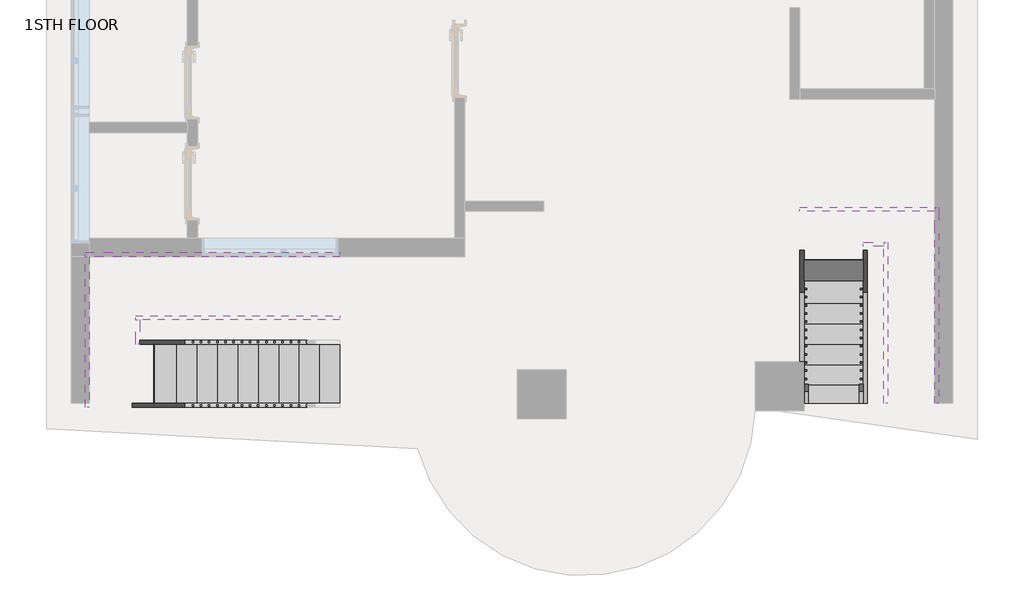
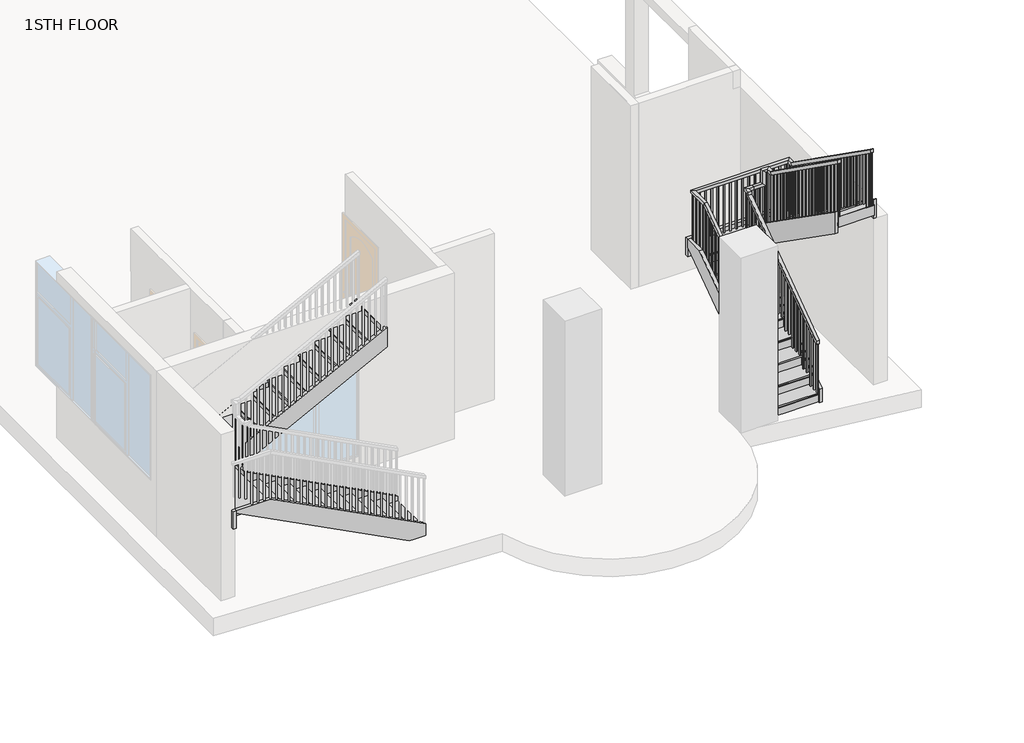
# One storey, part 4 of 4: 12 members, 2 railings, 2 stair flights.
"""IFC4 building model written with IfcOpenShell, lengths in millimetres."""

from ifc_helpers import new_model, si_unit, frame, origin, place, context, project, spatial, polyline, outline, extrude, faceted_brep, transform, mapped, element, save
from components import stair_flight_8de044e6, stair_flight_1dbbfd26

model = new_model("IFC4")

# Units and contexts
model_context = context("Model", 3, world=origin())
ifc_project = project(units=[si_unit("LENGTHUNIT", "METRE", prefix="MILLI")], contexts=[model_context])

# Site, building, storey
site = spatial("IfcSite", under=ifc_project)
building = spatial("IfcBuilding", under=site)
storey = spatial("IfcBuildingStorey", under=building, Name="1STH FLOOR", Elevation=3200.4)

# Members
placement = place(None, origin())
element("IfcMember", 1, ObjectType="Stringer - 2\" Width", at=placement, inside=storey, context=model_context, shape_type="SweptSolid", body=[
    extrude(outline(polyline([(3200.4, -3117.2664982), (3404.9197081, -3117.2664982), (4724.4, -5663.6319738), (4724.4, -6232.5131972), (4675.8929835, -6232.5131972), (3200.4, -3385.0705974), (3200.4, -3117.2664982)])), frame((0.0, -7701.7822004, 0.0), z_axis=(0.0, 1.0, 0.0), x_axis=(0.0, 0.0, 1.0)), (0.0, 0.0, 1.0), 50.8),
])
element("IfcMember", 2, ObjectType="Stringer - 2\" Width", at=placement, inside=storey, context=model_context, shape_type="SweptSolid", body=[
    extrude(outline(polyline([(-6232.5131972, -7701.7822004), (-6283.3131972, -7701.7822004), (-6283.3131972, -5824.7082131), (-6232.5131972, -5824.7082131), (-6232.5131972, -7701.7822004)])), frame((0.0, 0.0, 4419.6), z_axis=(0.0, 0.0, 1.0), x_axis=(1.0, 0.0, 0.0)), (0.0, 0.0, 1.0), 304.8),
])
element("IfcMember", 3, ObjectType="Stringer - 2\" Width", at=placement, inside=storey, context=model_context, shape_type="SweptSolid", body=[
    extrude(outline(polyline([(4528.3136913, -6283.3131972), (4419.6, -6283.3131972), (4419.6, -5830.6202937), (5825.6106031, -3117.2664982), (6168.9015263, -3117.2664982), (4528.3136913, -6283.3131972)])), frame((0.0, -5824.7082131, 0.0), z_axis=(0.0, 1.0, 0.0), x_axis=(0.0, 0.0, 1.0)), (0.0, 0.0, 1.0), 50.8),
])
element("IfcMember", 4, ObjectType="Stringer - 2\" Width", at=placement, inside=storey, context=model_context, shape_type="SweptSolid", body=[
    extrude(outline(polyline([(3200.4, -3117.2664982), (3404.9197081, -3117.2664982), (4694.7778899, -5606.4664982), (4351.4869668, -5606.4664982), (3200.4, -3385.0705974), (3200.4, -3117.2664982)])), frame((0.0, -6914.3822004, 0.0), z_axis=(0.0, 1.0, 0.0), x_axis=(0.0, 0.0, 1.0)), (0.0, 0.0, 1.0), 50.8),
])
element("IfcMember", 5, ObjectType="Stringer - 2\" Width", at=placement, inside=storey, context=model_context, shape_type="SweptSolid", body=[
    extrude(outline(polyline([(-5606.4664982, -6914.3822004), (-5657.2664982, -6914.3822004), (-5657.2664982, -6609.5822004), (-5606.4664982, -6609.5822004), (-5606.4664982, -6914.3822004)])), frame((0.0, 0.0, 4419.6), z_axis=(0.0, 0.0, 1.0), x_axis=(1.0, 0.0, 0.0)), (0.0, 0.0, 1.0), 304.8),
])
element("IfcMember", 6, ObjectType="Stringer - 2\" Width", at=placement, inside=storey, context=model_context, shape_type="SweptSolid", body=[
    extrude(outline(polyline([(4852.7197081, -5657.2664982), (4509.4287849, -5657.2664982), (5825.6106031, -3117.2664982), (6168.9015263, -3117.2664982), (4852.7197081, -5657.2664982)])), frame((0.0, -6609.5822004, 0.0), z_axis=(0.0, 1.0, 0.0), x_axis=(0.0, 0.0, 1.0)), (0.0, 0.0, 1.0), 50.8),
])
element("IfcMember", 7, ObjectType="Stringer - 2\" Width", at=placement, inside=storey, context=model_context, shape_type="SweptSolid", body=[
    extrude(outline(polyline([(-7650.9822004, 3200.4), (-7650.9822004, 3439.699187), (-5597.981039, 4876.8), (-5263.3822004, 4876.8), (-5263.3822004, 4738.9633718), (-7461.3298744, 3200.4), (-7650.9822004, 3200.4)])), frame((2606.6891134, 0.0, 0.0), z_axis=(1.0, 0.0, 0.0), x_axis=(0.0, 1.0, 0.0)), (0.0, 0.0, 1.0), 50.8),
])
element("IfcMember", 8, ObjectType="Stringer - 2\" Width", at=placement, inside=storey, context=model_context, shape_type="SweptSolid", body=[
    extrude(outline(polyline([(2606.6891134, -5263.3822004), (2606.6891134, -5212.5822004), (4281.7311655, -5212.5822004), (4281.7311655, -5263.3822004), (2606.6891134, -5263.3822004)])), frame((0.0, 0.0, 4572.0), z_axis=(0.0, 0.0, 1.0), x_axis=(1.0, 0.0, 0.0)), (0.0, 0.0, 1.0), 304.8),
])
element("IfcMember", 9, ObjectType="Stringer - 2\" Width", at=placement, inside=storey, context=model_context, shape_type="SweptSolid", body=[
    extrude(outline(polyline([(-5212.5822004, 4719.859187), (-5212.5822004, 4572.0), (-5532.8630978, 4572.0), (-7650.9822004, 6054.6833718), (-7650.9822004, 6426.739187), (-5212.5822004, 4719.859187)])), frame((4281.7311655, 0.0, 0.0), z_axis=(1.0, 0.0, 0.0), x_axis=(0.0, 1.0, 0.0)), (0.0, 0.0, 1.0), 50.8),
])
element("IfcMember", 10, ObjectType="Stringer - 2\" Width", at=placement, inside=storey, context=model_context, shape_type="SweptSolid", body=[
    extrude(outline(polyline([(-7650.9822004, 3200.4), (-7650.9822004, 3439.699187), (-5695.1822004, 4808.759187), (-5695.1822004, 4436.7033718), (-7461.3298744, 3200.4), (-7650.9822004, 3200.4)])), frame((3394.0891134, 0.0, 0.0), z_axis=(1.0, 0.0, 0.0), x_axis=(0.0, 1.0, 0.0)), (0.0, 0.0, 1.0), 50.8),
])
element("IfcMember", 11, ObjectType="Stringer - 2\" Width", at=placement, inside=storey, context=model_context, shape_type="SweptSolid", body=[
    extrude(outline(polyline([(3394.0891134, -5695.1822004), (3394.0891134, -5644.3822004), (3648.0891134, -5644.3822004), (3648.0891134, -5695.1822004), (3394.0891134, -5695.1822004)])), frame((0.0, 0.0, 4572.0), z_axis=(0.0, 0.0, 1.0), x_axis=(1.0, 0.0, 0.0)), (0.0, 0.0, 1.0), 304.8),
])
element("IfcMember", 12, ObjectType="Stringer - 2\" Width", at=placement, inside=storey, context=model_context, shape_type="SweptSolid", body=[
    extrude(outline(polyline([(-5644.3822004, 5022.119187), (-5644.3822004, 4650.0633718), (-7650.9822004, 6054.6833718), (-7650.9822004, 6426.739187), (-5644.3822004, 5022.119187)])), frame((3648.0891134, 0.0, 0.0), z_axis=(1.0, 0.0, 0.0), x_axis=(0.0, 1.0, 0.0)), (0.0, 0.0, 1.0), 50.8),
])

# Railings
element("IfcRailing", 13, ObjectType="Handrail - Rectangular", at=placement, inside=storey, context=model_context, shape_type="SolidModel", body=[
    faceted_brep([(3343.2891134, -7650.9822004, 4292.6), (3343.2891134, -7650.9822004, 4230.3314749), (3394.0891134, -7650.9822004, 4230.3314749), (3394.0891134, -7650.9822004, 4292.6), (3343.2891134, -5720.5822004, 5660.9848101), (3343.2891134, -5669.7822004, 5634.7264116), (3394.0891134, -5669.7822004, 5634.7264116), (3394.0891134, -5720.5822004, 5660.9848101), (3343.2891134, -5720.5822004, 5715.0), (3343.2891134, -5669.7822004, 5664.2), (3394.0891134, -5669.7822004, 5664.2), (3394.0891134, -5720.5822004, 5715.0), (3343.2891134, -5593.5822004, 5715.0), (3343.2891134, -5593.5822004, 5664.2), (3394.0891134, -5644.3822004, 5664.2), (3394.0891134, -5644.3822004, 5715.0), (3470.2891134, -5593.5822004, 5715.0), (3470.2891134, -5593.5822004, 5664.2), (3470.2891134, -5644.3822004, 5664.2), (3470.2891134, -5644.3822004, 5715.0), (3622.6891134, -5593.5822004, 5715.0), (3673.4891134, -5593.5822004, 5664.2), (3673.4891134, -5644.3822004, 5664.2), (3622.6891134, -5644.3822004, 5715.0), (3622.6891134, -5593.5822004, 5946.8151899), (3673.4891134, -5593.5822004, 5896.0151899), (3673.4891134, -5644.3822004, 5896.0151899), (3622.6891134, -5644.3822004, 5946.8151899), (3749.6891134, -5593.5822004, 5946.8151899), (3749.6891134, -5593.5822004, 5896.0151899), (3698.8891134, -5644.3822004, 5896.0151899), (3698.8891134, -5644.3822004, 5946.8151899), (3749.6891134, -5720.5822004, 5946.8151899), (3749.6891134, -5736.7610126, 5896.0151899), (3698.8891134, -5736.7610126, 5896.0151899), (3698.8891134, -5720.5822004, 5946.8151899), (3749.6891134, -7650.9822004, 7315.2), (3698.8891134, -7650.9822004, 7315.2), (3698.8891134, -7650.9822004, 7252.9314749), (3749.6891134, -7650.9822004, 7252.9314749)], [[[0, 1, 2, 3]], [[1, 0, 4, 5]], [[2, 1, 5, 6]], [[3, 2, 6, 7]], [[0, 3, 7, 4]], [[5, 4, 8, 9]], [[6, 5, 9, 10]], [[7, 6, 10, 11]], [[4, 7, 11, 8]], [[9, 8, 12, 13]], [[10, 9, 13, 14]], [[11, 10, 14, 15]], [[8, 11, 15, 12]], [[13, 12, 16, 17]], [[14, 13, 17, 18]], [[15, 14, 18, 19]], [[12, 15, 19, 16]], [[17, 16, 20, 21]], [[18, 17, 21, 22]], [[19, 18, 22, 23]], [[16, 19, 23, 20]], [[21, 20, 24, 25]], [[22, 21, 25, 26]], [[23, 22, 26, 27]], [[20, 23, 27, 24]], [[25, 24, 28, 29]], [[26, 25, 29, 30]], [[27, 26, 30, 31]], [[24, 27, 31, 28]], [[29, 28, 32, 33]], [[30, 29, 33, 34]], [[31, 30, 34, 35]], [[28, 31, 35, 32]], [[36, 37, 38, 39]], [[33, 32, 36, 39]], [[34, 33, 39, 38]], [[35, 34, 38, 37]], [[32, 35, 37, 36]]]),
    extrude(outline(polyline([(-7558.9072004, 7187.6631205), (-7539.8572004, 7174.159323), (-7539.8572004, 6223.0), (-7558.9072004, 6223.0), (-7558.9072004, 7187.6631205)])), frame((3714.7641134, 0.0, 0.0), z_axis=(1.0, 0.0, 0.0), x_axis=(0.0, 1.0, 0.0)), (0.0, 0.0, 1.0), 19.05),
    extrude(outline(polyline([(-7457.3072004, 7115.6428673), (-7438.2572004, 7102.1390699), (-7438.2572004, 6223.0), (-7457.3072004, 6223.0), (-7457.3072004, 7115.6428673)])), frame((3714.7641134, 0.0, 0.0), z_axis=(1.0, 0.0, 0.0), x_axis=(0.0, 1.0, 0.0)), (0.0, 0.0, 1.0), 19.05),
    extrude(outline(polyline([(-7355.7072004, 7043.6226142), (-7336.6572004, 7030.1188167), (-7336.6572004, 6045.2), (-7355.7072004, 6045.2), (-7355.7072004, 7043.6226142)])), frame((3714.7641134, 0.0, 0.0), z_axis=(1.0, 0.0, 0.0), x_axis=(0.0, 1.0, 0.0)), (0.0, 0.0, 1.0), 19.05),
    extrude(outline(polyline([(-7254.1072004, 6971.602361), (-7235.0572004, 6958.0985635), (-7235.0572004, 6045.2), (-7254.1072004, 6045.2), (-7254.1072004, 6971.602361)])), frame((3714.7641134, 0.0, 0.0), z_axis=(1.0, 0.0, 0.0), x_axis=(0.0, 1.0, 0.0)), (0.0, 0.0, 1.0), 19.05),
    extrude(outline(polyline([(-7152.5072004, 6899.5821078), (-7133.4572004, 6886.0783104), (-7133.4572004, 5867.4), (-7152.5072004, 5867.4), (-7152.5072004, 6899.5821078)])), frame((3714.7641134, 0.0, 0.0), z_axis=(1.0, 0.0, 0.0), x_axis=(0.0, 1.0, 0.0)), (0.0, 0.0, 1.0), 19.05),
    extrude(outline(polyline([(-7050.9072004, 6827.5618547), (-7031.8572004, 6814.0580572), (-7031.8572004, 5867.4), (-7050.9072004, 5867.4), (-7050.9072004, 6827.5618547)])), frame((3714.7641134, 0.0, 0.0), z_axis=(1.0, 0.0, 0.0), x_axis=(0.0, 1.0, 0.0)), (0.0, 0.0, 1.0), 19.05),
    extrude(outline(polyline([(-6949.3072004, 6755.5416015), (-6930.2572004, 6742.037804), (-6930.2572004, 5867.4), (-6949.3072004, 5867.4), (-6949.3072004, 6755.5416015)])), frame((3714.7641134, 0.0, 0.0), z_axis=(1.0, 0.0, 0.0), x_axis=(0.0, 1.0, 0.0)), (0.0, 0.0, 1.0), 19.05),
    extrude(outline(polyline([(-6847.7072004, 6683.5213483), (-6828.6572004, 6670.0175509), (-6828.6572004, 5689.6), (-6847.7072004, 5689.6), (-6847.7072004, 6683.5213483)])), frame((3714.7641134, 0.0, 0.0), z_axis=(1.0, 0.0, 0.0), x_axis=(0.0, 1.0, 0.0)), (0.0, 0.0, 1.0), 19.05),
    extrude(outline(polyline([(-6746.1072004, 6611.5010952), (-6727.0572004, 6597.9972977), (-6727.0572004, 5689.6), (-6746.1072004, 5689.6), (-6746.1072004, 6611.5010952)])), frame((3714.7641134, 0.0, 0.0), z_axis=(1.0, 0.0, 0.0), x_axis=(0.0, 1.0, 0.0)), (0.0, 0.0, 1.0), 19.05),
    extrude(outline(polyline([(-6644.5072004, 6539.480842), (-6625.4572004, 6525.9770445), (-6625.4572004, 5511.8), (-6644.5072004, 5511.8), (-6644.5072004, 6539.480842)])), frame((3714.7641134, 0.0, 0.0), z_axis=(1.0, 0.0, 0.0), x_axis=(0.0, 1.0, 0.0)), (0.0, 0.0, 1.0), 19.05),
    extrude(outline(polyline([(-6542.9072004, 6467.4605888), (-6523.8572004, 6453.9567914), (-6523.8572004, 5511.8), (-6542.9072004, 5511.8), (-6542.9072004, 6467.4605888)])), frame((3714.7641134, 0.0, 0.0), z_axis=(1.0, 0.0, 0.0), x_axis=(0.0, 1.0, 0.0)), (0.0, 0.0, 1.0), 19.05),
    extrude(outline(polyline([(-6441.3072004, 6395.4403357), (-6422.2572004, 6381.9365382), (-6422.2572004, 5511.8), (-6441.3072004, 5511.8), (-6441.3072004, 6395.4403357)])), frame((3714.7641134, 0.0, 0.0), z_axis=(1.0, 0.0, 0.0), x_axis=(0.0, 1.0, 0.0)), (0.0, 0.0, 1.0), 19.05),
    extrude(outline(polyline([(-6339.7072004, 6323.4200825), (-6320.6572004, 6309.916285), (-6320.6572004, 5334.0), (-6339.7072004, 5334.0), (-6339.7072004, 6323.4200825)])), frame((3714.7641134, 0.0, 0.0), z_axis=(1.0, 0.0, 0.0), x_axis=(0.0, 1.0, 0.0)), (0.0, 0.0, 1.0), 19.05),
    extrude(outline(polyline([(-6238.1072004, 6251.3998293), (-6219.0572004, 6237.8960319), (-6219.0572004, 5334.0), (-6238.1072004, 5334.0), (-6238.1072004, 6251.3998293)])), frame((3714.7641134, 0.0, 0.0), z_axis=(1.0, 0.0, 0.0), x_axis=(0.0, 1.0, 0.0)), (0.0, 0.0, 1.0), 19.05),
    extrude(outline(polyline([(-6136.5072004, 6179.3795762), (-6117.4572004, 6165.8757787), (-6117.4572004, 5156.2), (-6136.5072004, 5156.2), (-6136.5072004, 6179.3795762)])), frame((3714.7641134, 0.0, 0.0), z_axis=(1.0, 0.0, 0.0), x_axis=(0.0, 1.0, 0.0)), (0.0, 0.0, 1.0), 19.05),
    extrude(outline(polyline([(-6034.9072004, 6107.359323), (-6015.8572004, 6093.8555255), (-6015.8572004, 5156.2), (-6034.9072004, 5156.2), (-6034.9072004, 6107.359323)])), frame((3714.7641134, 0.0, 0.0), z_axis=(1.0, 0.0, 0.0), x_axis=(0.0, 1.0, 0.0)), (0.0, 0.0, 1.0), 19.05),
    extrude(outline(polyline([(-5933.3072004, 6035.3390699), (-5914.2572004, 6021.8352724), (-5914.2572004, 5156.2), (-5933.3072004, 5156.2), (-5933.3072004, 6035.3390699)])), frame((3714.7641134, 0.0, 0.0), z_axis=(1.0, 0.0, 0.0), x_axis=(0.0, 1.0, 0.0)), (0.0, 0.0, 1.0), 19.05),
    extrude(outline(polyline([(-5831.7072004, 5963.3188167), (-5812.6572004, 5949.8150192), (-5812.6572004, 4978.4), (-5831.7072004, 4978.4), (-5831.7072004, 5963.3188167)])), frame((3714.7641134, 0.0, 0.0), z_axis=(1.0, 0.0, 0.0), x_axis=(0.0, 1.0, 0.0)), (0.0, 0.0, 1.0), 19.05),
    extrude(outline(polyline([(-5730.1072004, 5891.2985635), (-5711.0572004, 5877.7947661), (-5711.0572004, 4978.4), (-5730.1072004, 4978.4), (-5730.1072004, 5891.2985635)])), frame((3714.7641134, 0.0, 0.0), z_axis=(1.0, 0.0, 0.0), x_axis=(0.0, 1.0, 0.0)), (0.0, 0.0, 1.0), 19.05),
    extrude(outline(polyline([(3663.9641134, -5628.5072004), (3663.9641134, -5609.4572004), (3683.0141134, -5609.4572004), (3683.0141134, -5628.5072004), (3663.9641134, -5628.5072004)])), frame((0.0, 0.0, 4800.6), z_axis=(0.0, 0.0, 1.0), x_axis=(1.0, 0.0, 0.0)), (0.0, 0.0, 1.0), 1095.4151899),
    extrude(outline(polyline([(3562.3641134, -5628.5072004), (3562.3641134, -5609.4572004), (3581.4141134, -5609.4572004), (3581.4141134, -5628.5072004), (3562.3641134, -5628.5072004)])), frame((0.0, 0.0, 4800.6), z_axis=(0.0, 0.0, 1.0), x_axis=(1.0, 0.0, 0.0)), (0.0, 0.0, 1.0), 863.6),
    extrude(outline(polyline([(3460.7641134, -5628.5072004), (3460.7641134, -5609.4572004), (3479.8141134, -5609.4572004), (3479.8141134, -5628.5072004), (3460.7641134, -5628.5072004)])), frame((0.0, 0.0, 4800.6), z_axis=(0.0, 0.0, 1.0), x_axis=(1.0, 0.0, 0.0)), (0.0, 0.0, 1.0), 863.6),
    extrude(outline(polyline([(-5730.1072004, 5591.9643863), (-5711.0572004, 5605.4681838), (-5711.0572004, 4622.8), (-5730.1072004, 4622.8), (-5730.1072004, 5591.9643863)])), frame((3359.1641134, 0.0, 0.0), z_axis=(1.0, 0.0, 0.0), x_axis=(0.0, 1.0, 0.0)), (0.0, 0.0, 1.0), 19.05),
    extrude(outline(polyline([(-5831.7072004, 5519.9441331), (-5812.6572004, 5533.4479306), (-5812.6572004, 4622.8), (-5831.7072004, 4622.8), (-5831.7072004, 5519.9441331)])), frame((3359.1641134, 0.0, 0.0), z_axis=(1.0, 0.0, 0.0), x_axis=(0.0, 1.0, 0.0)), (0.0, 0.0, 1.0), 19.05),
    extrude(outline(polyline([(-5933.3072004, 5447.92388), (-5914.2572004, 5461.4276774), (-5914.2572004, 4445.0), (-5933.3072004, 4445.0), (-5933.3072004, 5447.92388)])), frame((3359.1641134, 0.0, 0.0), z_axis=(1.0, 0.0, 0.0), x_axis=(0.0, 1.0, 0.0)), (0.0, 0.0, 1.0), 19.05),
    extrude(outline(polyline([(-6034.9072004, 5375.9036268), (-6015.8572004, 5389.4074243), (-6015.8572004, 4445.0), (-6034.9072004, 4445.0), (-6034.9072004, 5375.9036268)])), frame((3359.1641134, 0.0, 0.0), z_axis=(1.0, 0.0, 0.0), x_axis=(0.0, 1.0, 0.0)), (0.0, 0.0, 1.0), 19.05),
    extrude(outline(polyline([(-6136.5072004, 5303.8833736), (-6117.4572004, 5317.3871711), (-6117.4572004, 4445.0), (-6136.5072004, 4445.0), (-6136.5072004, 5303.8833736)])), frame((3359.1641134, 0.0, 0.0), z_axis=(1.0, 0.0, 0.0), x_axis=(0.0, 1.0, 0.0)), (0.0, 0.0, 1.0), 19.05),
    extrude(outline(polyline([(-6238.1072004, 5231.8631205), (-6219.0572004, 5245.366918), (-6219.0572004, 4267.2), (-6238.1072004, 4267.2), (-6238.1072004, 5231.8631205)])), frame((3359.1641134, 0.0, 0.0), z_axis=(1.0, 0.0, 0.0), x_axis=(0.0, 1.0, 0.0)), (0.0, 0.0, 1.0), 19.05),
    extrude(outline(polyline([(-6339.7072004, 5159.8428673), (-6320.6572004, 5173.3466648), (-6320.6572004, 4267.2), (-6339.7072004, 4267.2), (-6339.7072004, 5159.8428673)])), frame((3359.1641134, 0.0, 0.0), z_axis=(1.0, 0.0, 0.0), x_axis=(0.0, 1.0, 0.0)), (0.0, 0.0, 1.0), 19.05),
    extrude(outline(polyline([(-6441.3072004, 5087.8226142), (-6422.2572004, 5101.3264116), (-6422.2572004, 4089.4), (-6441.3072004, 4089.4), (-6441.3072004, 5087.8226142)])), frame((3359.1641134, 0.0, 0.0), z_axis=(1.0, 0.0, 0.0), x_axis=(0.0, 1.0, 0.0)), (0.0, 0.0, 1.0), 19.05),
    extrude(outline(polyline([(-6542.9072004, 5015.802361), (-6523.8572004, 5029.3061585), (-6523.8572004, 4089.4), (-6542.9072004, 4089.4), (-6542.9072004, 5015.802361)])), frame((3359.1641134, 0.0, 0.0), z_axis=(1.0, 0.0, 0.0), x_axis=(0.0, 1.0, 0.0)), (0.0, 0.0, 1.0), 19.05),
    extrude(outline(polyline([(-6644.5072004, 4943.7821078), (-6625.4572004, 4957.2859053), (-6625.4572004, 4089.4), (-6644.5072004, 4089.4), (-6644.5072004, 4943.7821078)])), frame((3359.1641134, 0.0, 0.0), z_axis=(1.0, 0.0, 0.0), x_axis=(0.0, 1.0, 0.0)), (0.0, 0.0, 1.0), 19.05),
    extrude(outline(polyline([(-6746.1072004, 4871.7618547), (-6727.0572004, 4885.2656521), (-6727.0572004, 3911.6), (-6746.1072004, 3911.6), (-6746.1072004, 4871.7618547)])), frame((3359.1641134, 0.0, 0.0), z_axis=(1.0, 0.0, 0.0), x_axis=(0.0, 1.0, 0.0)), (0.0, 0.0, 1.0), 19.05),
    extrude(outline(polyline([(-6847.7072004, 4799.7416015), (-6828.6572004, 4813.245399), (-6828.6572004, 3911.6), (-6847.7072004, 3911.6), (-6847.7072004, 4799.7416015)])), frame((3359.1641134, 0.0, 0.0), z_axis=(1.0, 0.0, 0.0), x_axis=(0.0, 1.0, 0.0)), (0.0, 0.0, 1.0), 19.05),
    extrude(outline(polyline([(-6949.3072004, 4727.7213483), (-6930.2572004, 4741.2251458), (-6930.2572004, 3733.8), (-6949.3072004, 3733.8), (-6949.3072004, 4727.7213483)])), frame((3359.1641134, 0.0, 0.0), z_axis=(1.0, 0.0, 0.0), x_axis=(0.0, 1.0, 0.0)), (0.0, 0.0, 1.0), 19.05),
    extrude(outline(polyline([(-7050.9072004, 4655.7010952), (-7031.8572004, 4669.2048926), (-7031.8572004, 3733.8), (-7050.9072004, 3733.8), (-7050.9072004, 4655.7010952)])), frame((3359.1641134, 0.0, 0.0), z_axis=(1.0, 0.0, 0.0), x_axis=(0.0, 1.0, 0.0)), (0.0, 0.0, 1.0), 19.05),
    extrude(outline(polyline([(-7152.5072004, 4583.680842), (-7133.4572004, 4597.1846395), (-7133.4572004, 3733.8), (-7152.5072004, 3733.8), (-7152.5072004, 4583.680842)])), frame((3359.1641134, 0.0, 0.0), z_axis=(1.0, 0.0, 0.0), x_axis=(0.0, 1.0, 0.0)), (0.0, 0.0, 1.0), 19.05),
    extrude(outline(polyline([(-7254.1072004, 4511.6605888), (-7235.0572004, 4525.1643863), (-7235.0572004, 3556.0), (-7254.1072004, 3556.0), (-7254.1072004, 4511.6605888)])), frame((3359.1641134, 0.0, 0.0), z_axis=(1.0, 0.0, 0.0), x_axis=(0.0, 1.0, 0.0)), (0.0, 0.0, 1.0), 19.05),
    extrude(outline(polyline([(-7355.7072004, 4439.6403357), (-7336.6572004, 4453.1441331), (-7336.6572004, 3556.0), (-7355.7072004, 3556.0), (-7355.7072004, 4439.6403357)])), frame((3359.1641134, 0.0, 0.0), z_axis=(1.0, 0.0, 0.0), x_axis=(0.0, 1.0, 0.0)), (0.0, 0.0, 1.0), 19.05),
    extrude(outline(polyline([(-7457.3072004, 4367.6200825), (-7438.2572004, 4381.12388), (-7438.2572004, 3378.2), (-7457.3072004, 3378.2), (-7457.3072004, 4367.6200825)])), frame((3359.1641134, 0.0, 0.0), z_axis=(1.0, 0.0, 0.0), x_axis=(0.0, 1.0, 0.0)), (0.0, 0.0, 1.0), 19.05),
    extrude(outline(polyline([(-7558.9072004, 4295.5998293), (-7539.8572004, 4309.1036268), (-7539.8572004, 3378.2), (-7558.9072004, 3378.2), (-7558.9072004, 4295.5998293)])), frame((3359.1641134, 0.0, 0.0), z_axis=(1.0, 0.0, 0.0), x_axis=(0.0, 1.0, 0.0)), (0.0, 0.0, 1.0), 19.05),
    extrude(outline(polyline([(3714.7641134, -5628.5072004), (3714.7641134, -5609.4572004), (3733.8141134, -5609.4572004), (3733.8141134, -5628.5072004), (3714.7641134, -5628.5072004)])), frame((0.0, 0.0, 4800.6), z_axis=(0.0, 0.0, 1.0), x_axis=(1.0, 0.0, 0.0)), (0.0, 0.0, 1.0), 1095.4151899),
    extrude(outline(polyline([(3378.2141134, -5628.5072004), (3359.1641134, -5628.5072004), (3359.1641134, -5609.4572004), (3378.2141134, -5609.4572004), (3378.2141134, -5628.5072004)])), frame((0.0, 0.0, 4800.6), z_axis=(0.0, 0.0, 1.0), x_axis=(1.0, 0.0, 0.0)), (0.0, 0.0, 1.0), 863.6),
    extrude(outline(polyline([(-7650.9822004, 7252.9314749), (-7631.9322004, 7239.4276774), (-7631.9322004, 6223.0), (-7650.9822004, 6223.0), (-7650.9822004, 7252.9314749)])), frame((3714.7641134, 0.0, 0.0), z_axis=(1.0, 0.0, 0.0), x_axis=(0.0, 1.0, 0.0)), (0.0, 0.0, 1.0), 19.05),
    extrude(outline(polyline([(-7650.9822004, 4230.3314749), (-7631.9322004, 4243.8352724), (-7631.9322004, 3378.2), (-7650.9822004, 3378.2), (-7650.9822004, 4230.3314749)])), frame((3359.1641134, 0.0, 0.0), z_axis=(1.0, 0.0, 0.0), x_axis=(0.0, 1.0, 0.0)), (0.0, 0.0, 1.0), 19.05),
])
element("IfcRailing", 14, ObjectType="Handrail - Rectangular", at=placement, inside=storey, context=model_context, shape_type="SolidModel", body=[
    faceted_brep([(2657.4891134, -7650.9822004, 4292.6), (2657.4891134, -7650.9822004, 4230.3314749), (2708.2891134, -7650.9822004, 4230.3314749), (2708.2891134, -7650.9822004, 4292.6), (2657.4891134, -5644.3822004, 5715.0), (2657.4891134, -5628.2033882, 5664.2), (2708.2891134, -5628.2033882, 5664.2), (2708.2891134, -5644.3822004, 5715.0), (2657.4891134, -5263.3822004, 5715.0), (2657.4891134, -5263.3822004, 5664.2), (2708.2891134, -5314.1822004, 5664.2), (2708.2891134, -5314.1822004, 5715.0), (4281.7311655, -5263.3822004, 5715.0), (4281.7311655, -5263.3822004, 5664.2), (4230.9311655, -5314.1822004, 5664.2), (4230.9311655, -5314.1822004, 5715.0), (4281.7311655, -5393.5572004, 5715.0), (4281.7311655, -5409.7360126, 5664.2), (4230.9311655, -5409.7360126, 5664.2), (4230.9311655, -5393.5572004, 5715.0), (4281.7311655, -7650.9822004, 7315.2), (4230.9311655, -7650.9822004, 7315.2), (4230.9311655, -7650.9822004, 7252.9314749), (4281.7311655, -7650.9822004, 7252.9314749)], [[[0, 1, 2, 3]], [[1, 0, 4, 5]], [[2, 1, 5, 6]], [[3, 2, 6, 7]], [[0, 3, 7, 4]], [[5, 4, 8, 9]], [[6, 5, 9, 10]], [[7, 6, 10, 11]], [[4, 7, 11, 8]], [[9, 8, 12, 13]], [[10, 9, 13, 14]], [[11, 10, 14, 15]], [[8, 11, 15, 12]], [[13, 12, 16, 17]], [[14, 13, 17, 18]], [[15, 14, 18, 19]], [[12, 15, 19, 16]], [[20, 21, 22, 23]], [[17, 16, 20, 23]], [[18, 17, 23, 22]], [[19, 18, 22, 21]], [[16, 19, 21, 20]]]),
    extrude(outline(polyline([(-7616.0572004, 7228.1745129), (-7616.0572004, 6223.0), (-7635.1072004, 6223.0), (-7635.1072004, 7241.6783104), (-7616.0572004, 7228.1745129)])), frame((4246.8061655, 0.0, 0.0), z_axis=(1.0, 0.0, 0.0), x_axis=(0.0, 1.0, 0.0)), (0.0, 0.0, 1.0), 19.05),
    extrude(outline(polyline([(-7514.4572004, 7156.1542597), (-7514.4572004, 6223.0), (-7533.5072004, 6223.0), (-7533.5072004, 7169.6580572), (-7514.4572004, 7156.1542597)])), frame((4246.8061655, 0.0, 0.0), z_axis=(1.0, 0.0, 0.0), x_axis=(0.0, 1.0, 0.0)), (0.0, 0.0, 1.0), 19.05),
    extrude(outline(polyline([(-7412.8572004, 7084.1340066), (-7412.8572004, 6223.0), (-7431.9072004, 6223.0), (-7431.9072004, 7097.637804), (-7412.8572004, 7084.1340066)])), frame((4246.8061655, 0.0, 0.0), z_axis=(1.0, 0.0, 0.0), x_axis=(0.0, 1.0, 0.0)), (0.0, 0.0, 1.0), 19.05),
    extrude(outline(polyline([(-7311.2572004, 7012.1137534), (-7311.2572004, 6045.2), (-7330.3072004, 6045.2), (-7330.3072004, 7025.6175509), (-7311.2572004, 7012.1137534)])), frame((4246.8061655, 0.0, 0.0), z_axis=(1.0, 0.0, 0.0), x_axis=(0.0, 1.0, 0.0)), (0.0, 0.0, 1.0), 19.05),
    extrude(outline(polyline([(-7209.6572004, 6940.0935002), (-7209.6572004, 6045.2), (-7228.7072004, 6045.2), (-7228.7072004, 6953.5972977), (-7209.6572004, 6940.0935002)])), frame((4246.8061655, 0.0, 0.0), z_axis=(1.0, 0.0, 0.0), x_axis=(0.0, 1.0, 0.0)), (0.0, 0.0, 1.0), 19.05),
    extrude(outline(polyline([(-7108.0572004, 6868.0732471), (-7108.0572004, 5867.4), (-7127.1072004, 5867.4), (-7127.1072004, 6881.5770445), (-7108.0572004, 6868.0732471)])), frame((4246.8061655, 0.0, 0.0), z_axis=(1.0, 0.0, 0.0), x_axis=(0.0, 1.0, 0.0)), (0.0, 0.0, 1.0), 19.05),
    extrude(outline(polyline([(-7006.4572004, 6796.0529939), (-7006.4572004, 5867.4), (-7025.5072004, 5867.4), (-7025.5072004, 6809.5567914), (-7006.4572004, 6796.0529939)])), frame((4246.8061655, 0.0, 0.0), z_axis=(1.0, 0.0, 0.0), x_axis=(0.0, 1.0, 0.0)), (0.0, 0.0, 1.0), 19.05),
    extrude(outline(polyline([(-6904.8572004, 6724.0327407), (-6904.8572004, 5867.4), (-6923.9072004, 5867.4), (-6923.9072004, 6737.5365382), (-6904.8572004, 6724.0327407)])), frame((4246.8061655, 0.0, 0.0), z_axis=(1.0, 0.0, 0.0), x_axis=(0.0, 1.0, 0.0)), (0.0, 0.0, 1.0), 19.05),
    extrude(outline(polyline([(-6803.2572004, 6652.0124876), (-6803.2572004, 5689.6), (-6822.3072004, 5689.6), (-6822.3072004, 6665.516285), (-6803.2572004, 6652.0124876)])), frame((4246.8061655, 0.0, 0.0), z_axis=(1.0, 0.0, 0.0), x_axis=(0.0, 1.0, 0.0)), (0.0, 0.0, 1.0), 19.05),
    extrude(outline(polyline([(-6701.6572004, 6579.9922344), (-6701.6572004, 5689.6), (-6720.7072004, 5689.6), (-6720.7072004, 6593.4960319), (-6701.6572004, 6579.9922344)])), frame((4246.8061655, 0.0, 0.0), z_axis=(1.0, 0.0, 0.0), x_axis=(0.0, 1.0, 0.0)), (0.0, 0.0, 1.0), 19.05),
    extrude(outline(polyline([(-6600.0572004, 6507.9719812), (-6600.0572004, 5511.8), (-6619.1072004, 5511.8), (-6619.1072004, 6521.4757787), (-6600.0572004, 6507.9719812)])), frame((4246.8061655, 0.0, 0.0), z_axis=(1.0, 0.0, 0.0), x_axis=(0.0, 1.0, 0.0)), (0.0, 0.0, 1.0), 19.05),
    extrude(outline(polyline([(-6498.4572004, 6435.9517281), (-6498.4572004, 5511.8), (-6517.5072004, 5511.8), (-6517.5072004, 6449.4555255), (-6498.4572004, 6435.9517281)])), frame((4246.8061655, 0.0, 0.0), z_axis=(1.0, 0.0, 0.0), x_axis=(0.0, 1.0, 0.0)), (0.0, 0.0, 1.0), 19.05),
    extrude(outline(polyline([(-6396.8572004, 6363.9314749), (-6396.8572004, 5511.8), (-6415.9072004, 5511.8), (-6415.9072004, 6377.4352724), (-6396.8572004, 6363.9314749)])), frame((4246.8061655, 0.0, 0.0), z_axis=(1.0, 0.0, 0.0), x_axis=(0.0, 1.0, 0.0)), (0.0, 0.0, 1.0), 19.05),
    extrude(outline(polyline([(-6295.2572004, 6291.9112217), (-6295.2572004, 5334.0), (-6314.3072004, 5334.0), (-6314.3072004, 6305.4150192), (-6295.2572004, 6291.9112217)])), frame((4246.8061655, 0.0, 0.0), z_axis=(1.0, 0.0, 0.0), x_axis=(0.0, 1.0, 0.0)), (0.0, 0.0, 1.0), 19.05),
    extrude(outline(polyline([(-6193.6572004, 6219.8909686), (-6193.6572004, 5334.0), (-6212.7072004, 5334.0), (-6212.7072004, 6233.3947661), (-6193.6572004, 6219.8909686)])), frame((4246.8061655, 0.0, 0.0), z_axis=(1.0, 0.0, 0.0), x_axis=(0.0, 1.0, 0.0)), (0.0, 0.0, 1.0), 19.05),
    extrude(outline(polyline([(-6092.0572004, 6147.8707154), (-6092.0572004, 5156.2), (-6111.1072004, 5156.2), (-6111.1072004, 6161.3745129), (-6092.0572004, 6147.8707154)])), frame((4246.8061655, 0.0, 0.0), z_axis=(1.0, 0.0, 0.0), x_axis=(0.0, 1.0, 0.0)), (0.0, 0.0, 1.0), 19.05),
    extrude(outline(polyline([(-5990.4572004, 6075.8504623), (-5990.4572004, 5156.2), (-6009.5072004, 5156.2), (-6009.5072004, 6089.3542597), (-5990.4572004, 6075.8504623)])), frame((4246.8061655, 0.0, 0.0), z_axis=(1.0, 0.0, 0.0), x_axis=(0.0, 1.0, 0.0)), (0.0, 0.0, 1.0), 19.05),
    extrude(outline(polyline([(-5888.8572004, 6003.8302091), (-5888.8572004, 5156.2), (-5907.9072004, 5156.2), (-5907.9072004, 6017.3340066), (-5888.8572004, 6003.8302091)])), frame((4246.8061655, 0.0, 0.0), z_axis=(1.0, 0.0, 0.0), x_axis=(0.0, 1.0, 0.0)), (0.0, 0.0, 1.0), 19.05),
    extrude(outline(polyline([(-5787.2572004, 5931.8099559), (-5787.2572004, 4978.4), (-5806.3072004, 4978.4), (-5806.3072004, 5945.3137534), (-5787.2572004, 5931.8099559)])), frame((4246.8061655, 0.0, 0.0), z_axis=(1.0, 0.0, 0.0), x_axis=(0.0, 1.0, 0.0)), (0.0, 0.0, 1.0), 19.05),
    extrude(outline(polyline([(-5685.6572004, 5859.7897028), (-5685.6572004, 4978.4), (-5704.7072004, 4978.4), (-5704.7072004, 5873.2935002), (-5685.6572004, 5859.7897028)])), frame((4246.8061655, 0.0, 0.0), z_axis=(1.0, 0.0, 0.0), x_axis=(0.0, 1.0, 0.0)), (0.0, 0.0, 1.0), 19.05),
    extrude(outline(polyline([(-5584.0572004, 5787.7694496), (-5584.0572004, 4800.6), (-5603.1072004, 4800.6), (-5603.1072004, 5801.2732471), (-5584.0572004, 5787.7694496)])), frame((4246.8061655, 0.0, 0.0), z_axis=(1.0, 0.0, 0.0), x_axis=(0.0, 1.0, 0.0)), (0.0, 0.0, 1.0), 19.05),
    extrude(outline(polyline([(-5482.4572004, 5715.7491964), (-5482.4572004, 4800.6), (-5501.5072004, 4800.6), (-5501.5072004, 5729.2529939), (-5482.4572004, 5715.7491964)])), frame((4246.8061655, 0.0, 0.0), z_axis=(1.0, 0.0, 0.0), x_axis=(0.0, 1.0, 0.0)), (0.0, 0.0, 1.0), 19.05),
    extrude(outline(polyline([(4265.8561655, -5380.8572004), (4265.8561655, -5399.9072004), (4246.8061655, -5399.9072004), (4246.8061655, -5380.8572004), (4265.8561655, -5380.8572004)])), frame((0.0, 0.0, 4800.6), z_axis=(0.0, 0.0, 1.0), x_axis=(1.0, 0.0, 0.0)), (0.0, 0.0, 1.0), 863.6),
    extrude(outline(polyline([(4197.3641134, -5279.2572004), (4216.4141134, -5279.2572004), (4216.4141134, -5298.3072004), (4197.3641134, -5298.3072004), (4197.3641134, -5279.2572004)])), frame((0.0, 0.0, 4800.6), z_axis=(0.0, 0.0, 1.0), x_axis=(1.0, 0.0, 0.0)), (0.0, 0.0, 1.0), 863.6),
    extrude(outline(polyline([(4095.7641134, -5279.2572004), (4114.8141134, -5279.2572004), (4114.8141134, -5298.3072004), (4095.7641134, -5298.3072004), (4095.7641134, -5279.2572004)])), frame((0.0, 0.0, 4800.6), z_axis=(0.0, 0.0, 1.0), x_axis=(1.0, 0.0, 0.0)), (0.0, 0.0, 1.0), 863.6),
    extrude(outline(polyline([(3994.1641134, -5279.2572004), (4013.2141134, -5279.2572004), (4013.2141134, -5298.3072004), (3994.1641134, -5298.3072004), (3994.1641134, -5279.2572004)])), frame((0.0, 0.0, 4800.6), z_axis=(0.0, 0.0, 1.0), x_axis=(1.0, 0.0, 0.0)), (0.0, 0.0, 1.0), 863.6),
    extrude(outline(polyline([(3892.5641134, -5279.2572004), (3911.6141134, -5279.2572004), (3911.6141134, -5298.3072004), (3892.5641134, -5298.3072004), (3892.5641134, -5279.2572004)])), frame((0.0, 0.0, 4800.6), z_axis=(0.0, 0.0, 1.0), x_axis=(1.0, 0.0, 0.0)), (0.0, 0.0, 1.0), 863.6),
    extrude(outline(polyline([(3790.9641134, -5279.2572004), (3810.0141134, -5279.2572004), (3810.0141134, -5298.3072004), (3790.9641134, -5298.3072004), (3790.9641134, -5279.2572004)])), frame((0.0, 0.0, 4800.6), z_axis=(0.0, 0.0, 1.0), x_axis=(1.0, 0.0, 0.0)), (0.0, 0.0, 1.0), 863.6),
    extrude(outline(polyline([(3689.3641134, -5279.2572004), (3708.4141134, -5279.2572004), (3708.4141134, -5298.3072004), (3689.3641134, -5298.3072004), (3689.3641134, -5279.2572004)])), frame((0.0, 0.0, 4800.6), z_axis=(0.0, 0.0, 1.0), x_axis=(1.0, 0.0, 0.0)), (0.0, 0.0, 1.0), 863.6),
    extrude(outline(polyline([(3587.7641134, -5279.2572004), (3606.8141134, -5279.2572004), (3606.8141134, -5298.3072004), (3587.7641134, -5298.3072004), (3587.7641134, -5279.2572004)])), frame((0.0, 0.0, 4800.6), z_axis=(0.0, 0.0, 1.0), x_axis=(1.0, 0.0, 0.0)), (0.0, 0.0, 1.0), 863.6),
    extrude(outline(polyline([(3486.1641134, -5279.2572004), (3505.2141134, -5279.2572004), (3505.2141134, -5298.3072004), (3486.1641134, -5298.3072004), (3486.1641134, -5279.2572004)])), frame((0.0, 0.0, 4800.6), z_axis=(0.0, 0.0, 1.0), x_axis=(1.0, 0.0, 0.0)), (0.0, 0.0, 1.0), 863.6),
    extrude(outline(polyline([(3384.5641134, -5279.2572004), (3403.6141134, -5279.2572004), (3403.6141134, -5298.3072004), (3384.5641134, -5298.3072004), (3384.5641134, -5279.2572004)])), frame((0.0, 0.0, 4800.6), z_axis=(0.0, 0.0, 1.0), x_axis=(1.0, 0.0, 0.0)), (0.0, 0.0, 1.0), 863.6),
    extrude(outline(polyline([(3282.9641134, -5279.2572004), (3302.0141134, -5279.2572004), (3302.0141134, -5298.3072004), (3282.9641134, -5298.3072004), (3282.9641134, -5279.2572004)])), frame((0.0, 0.0, 4800.6), z_axis=(0.0, 0.0, 1.0), x_axis=(1.0, 0.0, 0.0)), (0.0, 0.0, 1.0), 863.6),
    extrude(outline(polyline([(3181.3641134, -5279.2572004), (3200.4141134, -5279.2572004), (3200.4141134, -5298.3072004), (3181.3641134, -5298.3072004), (3181.3641134, -5279.2572004)])), frame((0.0, 0.0, 4800.6), z_axis=(0.0, 0.0, 1.0), x_axis=(1.0, 0.0, 0.0)), (0.0, 0.0, 1.0), 863.6),
    extrude(outline(polyline([(3079.7641134, -5279.2572004), (3098.8141134, -5279.2572004), (3098.8141134, -5298.3072004), (3079.7641134, -5298.3072004), (3079.7641134, -5279.2572004)])), frame((0.0, 0.0, 4800.6), z_axis=(0.0, 0.0, 1.0), x_axis=(1.0, 0.0, 0.0)), (0.0, 0.0, 1.0), 863.6),
    extrude(outline(polyline([(2978.1641134, -5279.2572004), (2997.2141134, -5279.2572004), (2997.2141134, -5298.3072004), (2978.1641134, -5298.3072004), (2978.1641134, -5279.2572004)])), frame((0.0, 0.0, 4800.6), z_axis=(0.0, 0.0, 1.0), x_axis=(1.0, 0.0, 0.0)), (0.0, 0.0, 1.0), 863.6),
    extrude(outline(polyline([(2876.5641134, -5279.2572004), (2895.6141134, -5279.2572004), (2895.6141134, -5298.3072004), (2876.5641134, -5298.3072004), (2876.5641134, -5279.2572004)])), frame((0.0, 0.0, 4800.6), z_axis=(0.0, 0.0, 1.0), x_axis=(1.0, 0.0, 0.0)), (0.0, 0.0, 1.0), 863.6),
    extrude(outline(polyline([(2774.9641134, -5279.2572004), (2794.0141134, -5279.2572004), (2794.0141134, -5298.3072004), (2774.9641134, -5298.3072004), (2774.9641134, -5279.2572004)])), frame((0.0, 0.0, 4800.6), z_axis=(0.0, 0.0, 1.0), x_axis=(1.0, 0.0, 0.0)), (0.0, 0.0, 1.0), 863.6),
    extrude(outline(polyline([(2673.3641134, -5323.7072004), (2673.3641134, -5304.6572004), (2692.4141134, -5304.6572004), (2692.4141134, -5323.7072004), (2673.3641134, -5323.7072004)])), frame((0.0, 0.0, 4800.6), z_axis=(0.0, 0.0, 1.0), x_axis=(1.0, 0.0, 0.0)), (0.0, 0.0, 1.0), 863.6),
    extrude(outline(polyline([(2673.3641134, -5425.3072004), (2673.3641134, -5406.2572004), (2692.4141134, -5406.2572004), (2692.4141134, -5425.3072004), (2673.3641134, -5425.3072004)])), frame((0.0, 0.0, 4800.6), z_axis=(0.0, 0.0, 1.0), x_axis=(1.0, 0.0, 0.0)), (0.0, 0.0, 1.0), 863.6),
    extrude(outline(polyline([(2673.3641134, -5526.9072004), (2673.3641134, -5507.8572004), (2692.4141134, -5507.8572004), (2692.4141134, -5526.9072004), (2673.3641134, -5526.9072004)])), frame((0.0, 0.0, 4800.6), z_axis=(0.0, 0.0, 1.0), x_axis=(1.0, 0.0, 0.0)), (0.0, 0.0, 1.0), 863.6),
    extrude(outline(polyline([(2673.3641134, -5628.5072004), (2673.3641134, -5609.4572004), (2692.4141134, -5609.4572004), (2692.4141134, -5628.5072004), (2673.3641134, -5628.5072004)])), frame((0.0, 0.0, 4800.6), z_axis=(0.0, 0.0, 1.0), x_axis=(1.0, 0.0, 0.0)), (0.0, 0.0, 1.0), 863.6),
    extrude(outline(polyline([(-5711.0572004, 5605.4681838), (-5711.0572004, 4622.8), (-5730.1072004, 4622.8), (-5730.1072004, 5591.9643863), (-5711.0572004, 5605.4681838)])), frame((2673.3641134, 0.0, 0.0), z_axis=(1.0, 0.0, 0.0), x_axis=(0.0, 1.0, 0.0)), (0.0, 0.0, 1.0), 19.05),
    extrude(outline(polyline([(-5812.6572004, 5533.4479306), (-5812.6572004, 4622.8), (-5831.7072004, 4622.8), (-5831.7072004, 5519.9441331), (-5812.6572004, 5533.4479306)])), frame((2673.3641134, 0.0, 0.0), z_axis=(1.0, 0.0, 0.0), x_axis=(0.0, 1.0, 0.0)), (0.0, 0.0, 1.0), 19.05),
    extrude(outline(polyline([(-5914.2572004, 5461.4276774), (-5914.2572004, 4445.0), (-5933.3072004, 4445.0), (-5933.3072004, 5447.92388), (-5914.2572004, 5461.4276774)])), frame((2673.3641134, 0.0, 0.0), z_axis=(1.0, 0.0, 0.0), x_axis=(0.0, 1.0, 0.0)), (0.0, 0.0, 1.0), 19.05),
    extrude(outline(polyline([(-6015.8572004, 5389.4074243), (-6015.8572004, 4445.0), (-6034.9072004, 4445.0), (-6034.9072004, 5375.9036268), (-6015.8572004, 5389.4074243)])), frame((2673.3641134, 0.0, 0.0), z_axis=(1.0, 0.0, 0.0), x_axis=(0.0, 1.0, 0.0)), (0.0, 0.0, 1.0), 19.05),
    extrude(outline(polyline([(-6117.4572004, 5317.3871711), (-6117.4572004, 4445.0), (-6136.5072004, 4445.0), (-6136.5072004, 5303.8833736), (-6117.4572004, 5317.3871711)])), frame((2673.3641134, 0.0, 0.0), z_axis=(1.0, 0.0, 0.0), x_axis=(0.0, 1.0, 0.0)), (0.0, 0.0, 1.0), 19.05),
    extrude(outline(polyline([(-6219.0572004, 5245.366918), (-6219.0572004, 4267.2), (-6238.1072004, 4267.2), (-6238.1072004, 5231.8631205), (-6219.0572004, 5245.366918)])), frame((2673.3641134, 0.0, 0.0), z_axis=(1.0, 0.0, 0.0), x_axis=(0.0, 1.0, 0.0)), (0.0, 0.0, 1.0), 19.05),
    extrude(outline(polyline([(-6320.6572004, 5173.3466648), (-6320.6572004, 4267.2), (-6339.7072004, 4267.2), (-6339.7072004, 5159.8428673), (-6320.6572004, 5173.3466648)])), frame((2673.3641134, 0.0, 0.0), z_axis=(1.0, 0.0, 0.0), x_axis=(0.0, 1.0, 0.0)), (0.0, 0.0, 1.0), 19.05),
    extrude(outline(polyline([(-6422.2572004, 5101.3264116), (-6422.2572004, 4089.4), (-6441.3072004, 4089.4), (-6441.3072004, 5087.8226142), (-6422.2572004, 5101.3264116)])), frame((2673.3641134, 0.0, 0.0), z_axis=(1.0, 0.0, 0.0), x_axis=(0.0, 1.0, 0.0)), (0.0, 0.0, 1.0), 19.05),
    extrude(outline(polyline([(-6523.8572004, 5029.3061585), (-6523.8572004, 4089.4), (-6542.9072004, 4089.4), (-6542.9072004, 5015.802361), (-6523.8572004, 5029.3061585)])), frame((2673.3641134, 0.0, 0.0), z_axis=(1.0, 0.0, 0.0), x_axis=(0.0, 1.0, 0.0)), (0.0, 0.0, 1.0), 19.05),
    extrude(outline(polyline([(-6625.4572004, 4957.2859053), (-6625.4572004, 4089.4), (-6644.5072004, 4089.4), (-6644.5072004, 4943.7821078), (-6625.4572004, 4957.2859053)])), frame((2673.3641134, 0.0, 0.0), z_axis=(1.0, 0.0, 0.0), x_axis=(0.0, 1.0, 0.0)), (0.0, 0.0, 1.0), 19.05),
    extrude(outline(polyline([(-6727.0572004, 4885.2656521), (-6727.0572004, 3911.6), (-6746.1072004, 3911.6), (-6746.1072004, 4871.7618547), (-6727.0572004, 4885.2656521)])), frame((2673.3641134, 0.0, 0.0), z_axis=(1.0, 0.0, 0.0), x_axis=(0.0, 1.0, 0.0)), (0.0, 0.0, 1.0), 19.05),
    extrude(outline(polyline([(-6828.6572004, 4813.245399), (-6828.6572004, 3911.6), (-6847.7072004, 3911.6), (-6847.7072004, 4799.7416015), (-6828.6572004, 4813.245399)])), frame((2673.3641134, 0.0, 0.0), z_axis=(1.0, 0.0, 0.0), x_axis=(0.0, 1.0, 0.0)), (0.0, 0.0, 1.0), 19.05),
    extrude(outline(polyline([(-6930.2572004, 4741.2251458), (-6930.2572004, 3733.8), (-6949.3072004, 3733.8), (-6949.3072004, 4727.7213483), (-6930.2572004, 4741.2251458)])), frame((2673.3641134, 0.0, 0.0), z_axis=(1.0, 0.0, 0.0), x_axis=(0.0, 1.0, 0.0)), (0.0, 0.0, 1.0), 19.05),
    extrude(outline(polyline([(-7031.8572004, 4669.2048926), (-7031.8572004, 3733.8), (-7050.9072004, 3733.8), (-7050.9072004, 4655.7010952), (-7031.8572004, 4669.2048926)])), frame((2673.3641134, 0.0, 0.0), z_axis=(1.0, 0.0, 0.0), x_axis=(0.0, 1.0, 0.0)), (0.0, 0.0, 1.0), 19.05),
    extrude(outline(polyline([(-7133.4572004, 4597.1846395), (-7133.4572004, 3733.8), (-7152.5072004, 3733.8), (-7152.5072004, 4583.680842), (-7133.4572004, 4597.1846395)])), frame((2673.3641134, 0.0, 0.0), z_axis=(1.0, 0.0, 0.0), x_axis=(0.0, 1.0, 0.0)), (0.0, 0.0, 1.0), 19.05),
    extrude(outline(polyline([(-7235.0572004, 4525.1643863), (-7235.0572004, 3556.0), (-7254.1072004, 3556.0), (-7254.1072004, 4511.6605888), (-7235.0572004, 4525.1643863)])), frame((2673.3641134, 0.0, 0.0), z_axis=(1.0, 0.0, 0.0), x_axis=(0.0, 1.0, 0.0)), (0.0, 0.0, 1.0), 19.05),
    extrude(outline(polyline([(-7336.6572004, 4453.1441331), (-7336.6572004, 3556.0), (-7355.7072004, 3556.0), (-7355.7072004, 4439.6403357), (-7336.6572004, 4453.1441331)])), frame((2673.3641134, 0.0, 0.0), z_axis=(1.0, 0.0, 0.0), x_axis=(0.0, 1.0, 0.0)), (0.0, 0.0, 1.0), 19.05),
    extrude(outline(polyline([(-7438.2572004, 4381.12388), (-7438.2572004, 3378.2), (-7457.3072004, 3378.2), (-7457.3072004, 4367.6200825), (-7438.2572004, 4381.12388)])), frame((2673.3641134, 0.0, 0.0), z_axis=(1.0, 0.0, 0.0), x_axis=(0.0, 1.0, 0.0)), (0.0, 0.0, 1.0), 19.05),
    extrude(outline(polyline([(-7539.8572004, 4309.1036268), (-7539.8572004, 3378.2), (-7558.9072004, 3378.2), (-7558.9072004, 4295.5998293), (-7539.8572004, 4309.1036268)])), frame((2673.3641134, 0.0, 0.0), z_axis=(1.0, 0.0, 0.0), x_axis=(0.0, 1.0, 0.0)), (0.0, 0.0, 1.0), 19.05),
    extrude(outline(polyline([(4246.8061655, -5279.2572004), (4265.8561655, -5279.2572004), (4265.8561655, -5298.3072004), (4246.8061655, -5298.3072004), (4246.8061655, -5279.2572004)])), frame((0.0, 0.0, 4800.6), z_axis=(0.0, 0.0, 1.0), x_axis=(1.0, 0.0, 0.0)), (0.0, 0.0, 1.0), 863.6),
    extrude(outline(polyline([(2673.3641134, -5298.3072004), (2673.3641134, -5279.2572004), (2692.4141134, -5279.2572004), (2692.4141134, -5298.3072004), (2673.3641134, -5298.3072004)])), frame((0.0, 0.0, 4800.6), z_axis=(0.0, 0.0, 1.0), x_axis=(1.0, 0.0, 0.0)), (0.0, 0.0, 1.0), 863.6),
    extrude(outline(polyline([(-7631.9322004, 7239.4276774), (-7631.9322004, 6223.0), (-7650.9822004, 6223.0), (-7650.9822004, 7252.9314749), (-7631.9322004, 7239.4276774)])), frame((4246.8061655, 0.0, 0.0), z_axis=(1.0, 0.0, 0.0), x_axis=(0.0, 1.0, 0.0)), (0.0, 0.0, 1.0), 19.05),
    extrude(outline(polyline([(-7631.9322004, 4243.8352724), (-7631.9322004, 3378.2), (-7650.9822004, 3378.2), (-7650.9822004, 4230.3314749), (-7631.9322004, 4243.8352724)])), frame((2673.3641134, 0.0, 0.0), z_axis=(1.0, 0.0, 0.0), x_axis=(0.0, 1.0, 0.0)), (0.0, 0.0, 1.0), 19.05),
])

# Stair flights
stair_flight_shape = stair_flight_8de044e6(model_context)
element("IfcStairFlight", 15, ObjectType="2\" Tread 1\" Nosing 1/4\" Riser", at=placement, inside=storey, context=model_context, shape_type="MappedRepresentation", body=[
    mapped(stair_flight_shape, transform((0.0, 0.0, 0.0), x_axis=(1.0, 0.0, 0.0), y_axis=(0.0, 1.0, 0.0), z_axis=(0.0, 0.0, 1.0))),
])
stair_flight_2_shape = stair_flight_1dbbfd26(model_context)
element("IfcStairFlight", 16, ObjectType="2\" Tread 1\" Nosing 1/4\" Riser", at=placement, inside=storey, context=model_context, shape_type="MappedRepresentation", body=[
    mapped(stair_flight_2_shape, transform((0.0, 0.0, 0.0), x_axis=(1.0, 0.0, 0.0), y_axis=(0.0, 1.0, 0.0), z_axis=(0.0, 0.0, 1.0))),
])

save(model, "model.ifc")

# Revit data of these elements
# Type "Handrail - Rectangular"
#   Assembly Code = "C2010400"
#   built-in parameter 1008612 = 0.0416667 (stored number, unit not read)
#   built-in parameter 1008611 = 0.0416667 (stored number, unit not read)
#   built-in parameter 1008609 = 0.333333 (stored number, unit not read)
#   built-in parameter 1008604 = 0.166667 (stored number, unit not read)
#   built-in parameter 1008603 = 0.166667 (stored number, unit not read)
#   Railing Height = 3' - 0"
#   built-in parameter 1008630 = 2
#   built-in parameter 1008610 = 2
#   built-in parameter 1008618 = Baluster - Square : 3/4"
# Elements 1, 2, 3, 4, 5, 6, 7, 8, 9, 10, 11, 12 (IfcMember, "Stringer - 2\" Width")
#   Phase Created = New Construction
# Elements 13, 14 (IfcRailing, "Handrail - Rectangular")
#   Phase Created = New Construction
# Elements 15, 16 (IfcStairFlight, "2\" Tread 1\" Nosing 1/4\" Riser")
#   Phase Created = New Construction
